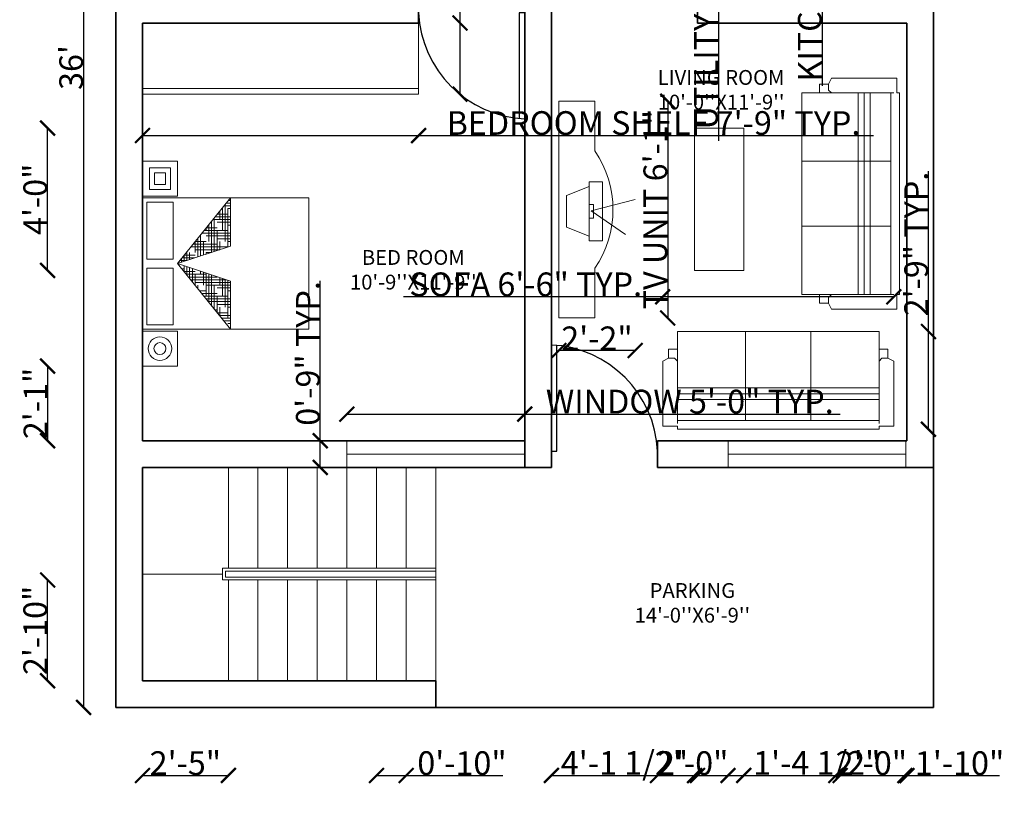
# Model space of a CAD drawing. Units: inches. Extents: x 2435 to 2891, y 1790 to 2334.
# Tile 1 of 3: x 2491 to 2823, y 1790 to 2052. Entities that reach past the tile are written whole.
import ezdxf

# ---------------------------------------------------------------- set-up
doc = ezdxf.new("R2010")
doc.units = ezdxf.units.IN
for name, color, linetype, lineweight in [('A-ANNO-DIMS', 2, 'Continuous', 13), ('A-AREA-IDEN', 7, 'Continuous', 18), ('A-FURN', 8, 'Continuous', 18), ('DOOR', 30, 'Continuous', 25), ('SHELF', 140, 'Continuous', 18), ('STEPS', 50, 'Continuous', 18), ('WALL', 7, 'Continuous', 35), ('WINDOW', 170, 'Continuous', 18)]:
    doc.layers.add(name, color=color, linetype=linetype, lineweight=lineweight)
doc.styles.get("Standard").update_dxf_attribs({"font": 'arial.ttf'})
doc.dimstyles.get("Standard").update_dxf_attribs({"dimtxt": 8, "dimasz": 5, "dimexe": 0.18, "dimexo": 0.0625, "dimgap": 0.09, "dimtad": 1, "dimdec": 1, "dimzin": 0, "dimdsep": 46, "dimlunit": 4, "dimtxsty": 'Standard', "dimblk": 'ARCHTICK', "dimcen": 0.09, "dimse1": 1, "dimse2": 1, "dimadec": 0, "dimazin": 0, "dimtfac": 1, "dimtdec": 1, "dimtofl": 0, "dimtmove": 0, "dimatfit": 3, "dimfxl": 1, "dimtolj": 1, "dimtzin": 0, "dimarcsym": 0})

# ---------------------------------------------------------------- blocks, each defined once
blk = doc.blocks.new('*X3')
at = {"color": 0}
for p, q in [((20.149, 14.719), (20.277, 14.719)), ((20.156, 14.625), (20.156, 14.728)), ((20.174, 14.75), (20.277, 14.75)), ((20.188, 14.75), (20.188, 14.767)), ((20.199, 14.781), (20.277, 14.781)), ((20.25, 14.812), (20.277, 14.812)), ((20.25, 14.319), (20.25, 14.75)), ((20.062, 14.257), (20.062, 14.612)), ((20.094, 14.375), (20.094, 14.65)), ((20.098, 14.656), (20.125, 14.656)), ((20.124, 14.688), (20.25, 14.688)), ((20.125, 14.5), (20.125, 14.689)), ((20.219, 14.309), (20.219, 14.625)), ((20.25, 14.625), (20.277, 14.625)), ((19.973, 14.5), (20.25, 14.5)), ((19.998, 14.531), (20.277, 14.531)), ((20, 14.237), (20, 14.5)), ((20.023, 14.562), (20.277, 14.562)), ((20.031, 14.247), (20.031, 14.573)), ((20.125, 14.594), (20.277, 14.594)), ((20.188, 14.299), (20.188, 14.5)), ((19.906, 14.375), (19.906, 14.417)), ((19.922, 14.438), (20, 14.438)), ((19.948, 14.469), (20.125, 14.469)), ((20.125, 14.406), (20.277, 14.406)), ((20.25, 14.438), (20.277, 14.438)), ((19.797, 14.281), (20.125, 14.281)), ((19.812, 14.174), (19.812, 14.301)), ((19.822, 14.312), (20.229, 14.312)), ((19.844, 14.185), (19.844, 14.34)), ((19.875, 14.25), (19.875, 14.379)), ((19.875, 14.344), (20.277, 14.344)), ((19.969, 14.226), (19.969, 14.375)), ((20, 14.375), (20.277, 14.375)), ((20.156, 14.288), (20.156, 14.375)), ((19.721, 14.188), (19.75, 14.188)), ((19.746, 14.219), (19.875, 14.219)), ((19.75, 14.154), (19.75, 14.223)), ((19.772, 14.25), (20, 14.25)), ((19.781, 14.164), (19.781, 14.262)), ((19.938, 14.216), (19.938, 14.25)), ((19.702, 14.094), (19.779, 14.094)), ((19.719, 14.073), (19.719, 14.114)), ((19.727, 14.062), (19.873, 14.062)), ((19.75, 14.034), (19.75, 14.103)), ((19.781, 13.995), (19.781, 14.093)), ((19.812, 14), (19.812, 14.082)), ((19.906, 13.84), (19.906, 14.051)), ((19.752, 14.031), (19.875, 14.031)), ((19.827, 13.938), (20.25, 13.938)), ((19.875, 13.878), (19.875, 14)), ((19.875, 13.969), (20.156, 13.969)), ((19.938, 13.801), (19.938, 14.041)), ((19.969, 13.875), (19.969, 14.031)), ((20, 14), (20, 14.02)), ((20, 14), (20.061, 14)), ((20.062, 13.645), (20.062, 14)), ((20.094, 13.625), (20.094, 13.989)), ((20.125, 13.75), (20.125, 13.979)), ((20.156, 13.875), (20.156, 13.969)), ((20.25, 13.5), (20.25, 13.937)), ((19.853, 13.906), (20.125, 13.906)), ((19.878, 13.875), (20, 13.875)), ((20.031, 13.684), (20.031, 13.875)), ((20.125, 13.844), (20.277, 13.844)), ((20.219, 13.451), (20.219, 13.875)), ((20.25, 13.875), (20.277, 13.875)), ((19.953, 13.781), (20.277, 13.781)), ((19.978, 13.75), (20.25, 13.75)), ((20, 13.812), (20.277, 13.812)), ((20, 13.723), (20, 13.75)), ((20.003, 13.719), (20.125, 13.719)), ((20.188, 13.49), (20.188, 13.75)), ((20.079, 13.625), (20.277, 13.625)), ((20.104, 13.594), (20.277, 13.594)), ((20.125, 13.656), (20.277, 13.656)), ((20.156, 13.529), (20.156, 13.625)), ((20.25, 13.688), (20.277, 13.688)), ((20.129, 13.562), (20.25, 13.562)), ((20.25, 13.5), (20.277, 13.5)), ((20.205, 13.469), (20.277, 13.469)), ((20.23, 13.438), (20.277, 13.438)), ((20.255, 13.406), (20.277, 13.406))]:
    blk.add_line(p, q, dxfattribs=at)
blk = doc.blocks.new('MAT-P13')
for p, q in [((-1.17, 0), (-1.17, -0.4)), ((-1.17, 0), (-0.77, 0)), ((-0.77, 0), (-0.77, -0.4)), ((-0.75, 0), (0.75, 0)), ((-0.75, 0), (-0.75, -1.9)), ((0.75, 0), (0.75, -1.9)), ((0.77, 0), (1.17, 0)), ((0.77, 0), (0.77, -0.4)), ((1.17, 0), (1.17, -0.4)), ((-0.7, -0.05), (-0.7, -0.35)), ((-0.7, -0.05), (-0.05, -0.05)), ((-0.05, -0.35), (-0.05, -0.05)), ((0.05, -0.05), (0.7, -0.05)), ((0.05, -0.35), (0.05, -0.05)), ((0.7, -0.05), (0.7, -0.35)), ((-1.17, -0.4), (-0.77, -0.4)), ((-0.75, -1.003), (0, -0.4)), ((0, -0.4), (-0.75, -1.003)), ((-0.7, -0.35), (-0.05, -0.35)), ((0, -0.4), (-0.2, -1.003)), ((0, -0.4), (0.2, -1.003)), ((0, -0.4), (0.75, -1.003)), ((0.05, -0.35), (0.7, -0.35)), ((0.77, -0.4), (1.17, -0.4)), ((-0.75, -1.003), (-0.2, -1.003)), ((0.2, -1.003), (0.75, -1.003)), ((0.75, -1.9), (-0.75, -1.9))]:
    blk.add_line(p, q)
for points in [[(0.847, -0.081), (1.093, -0.081), (1.093, -0.319), (0.847, -0.319)], [(0.902, -0.136), (1.038, -0.136), (1.038, -0.264), (0.902, -0.264)]]:
    blk.add_lwpolyline(points, close=True)
for radius in [0.134, 0.0686]:
    blk.add_circle((-0.97, -0.2), radius)
at = {"xscale": -1, "rotation": 90}
blk.add_blockref('*X3', (14.128, 19.274), dxfattribs=at)
blk = doc.blocks.new('12PCOU13')
at = {"color": 0, "linetype": 'ByBlock'}
for p, q in [((24, 37), (24, 35)), ((23, 34), (2, 34)), ((3, -34), (3, 34)), ((10, 34), (10, -34)), ((12, 34), (12, -34)), ((14, 34), (14, -34)), ((24, 35), (23, 34)), ((27, 34), (23, 34)), ((33, 11), (3, 11)), ((33, -11), (3, -11)), ((23, -34), (2, -34)), ((27, -34), (23, -34)), ((24, -35), (23, -34)), ((24, -37), (24, -35))]:
    blk.add_line(p, q, dxfattribs=at)
blk.add_lwpolyline([(1, -39), (1, -34), (0, -34), (0, 34), (1, 34), (1, 39), (23, 39), (24, 37), (27, 37), (27, 34), (33, 34), (33, -34), (27, -34), (27, -37), (24, -37), (23, -39)], close=True, dxfattribs=at)
blk = doc.blocks.new('AP0B05')
for p, q in [((35, 100), (35, 880)), ((75, 100), (75, 878.9)), ((35, 100), (35, -20)), ((815, 100), (815, -20))]:
    blk.add_line(p, q)
blk.add_lwpolyline([(35, 100), (75, 100)])
blk.add_arc((-2.4, 62.6), 818.3, 2.62122, 87.37878)
blk = doc.blocks.new('banghe81')
for p, q in [((-500, 3000), (0, 3000)), ((-500, 2312), (-500, 3000)), ((0, 3000), (0, 0)), ((-607, 1930), (-419, 1930)), ((-607, 1117), (-607, 1930)), ((-419, 1930), (-419, 1117)), ((-925, 1843), (-450, 1517)), ((-107, 1742), (-419, 1867)), ((-107, 1305), (-107, 1742)), ((-450, 1517), (-1057, 1361)), ((-482, 1617), (-482, 1430)), ((-419, 1617), (-482, 1617)), ((-482, 1430), (-419, 1430)), ((-419, 1180), (-107, 1305)), ((-419, 1117), (-607, 1117)), ((-500, 0), (-500, 688)), ((0, 0), (-500, 0)), ((-500, 0), (-500, 0))]:
    blk.add_line(p, q)
blk.add_arc((695, 1500), 1445, 145.7945, 214.2055)
blk = doc.blocks.new('_ArchTick')
at = {"color": 0, "linetype": 'ByBlock', "const_width": 0.15}
blk.add_lwpolyline([(-0.5, -0.5), (0.5, 0.5)], dxfattribs=at)
blk = doc.blocks.new('*D11')
at = {"layer": 'A-ANNO-DIMS', "color": 0, "lineweight": -2, "transparency": 16777216}
blk.add_line((2512.57, 2252.2), (2512.57, 1820.2), dxfattribs=at)
at = {"layer": 'Defpoints', "color": 0, "transparency": 16777216}
for p in [(2523.44, 2252.2), (2512.57, 1820.2), (2523.44, 1820.2)]:
    blk.add_point(p, dxfattribs=at)
at = {"layer": 'A-ANNO-DIMS', "color": 0, "lineweight": -2, "transparency": 16777216, "xscale": 5, "yscale": 5, "zscale": 5}
for p, rotation in [((2512.57, 2252.2), 90), ((2512.57, 1820.2), 270)]:
    blk.add_blockref('_ArchTick', p, dxfattribs=dict(at, rotation=rotation))
at = {"layer": 'A-ANNO-DIMS', "color": 0, "transparency": 16777216, "insert": (2508.39, 2036.2), "char_height": 8, "attachment_point": 5, "rotation": 90}
blk.add_mtext("\\A1;36'", dxfattribs=at)
blk = doc.blocks.new('WIN-60IN')
blk.add_line((0, 4.5), (60, 4.5))
blk.add_lwpolyline([(0, 9), (60, 9), (60, 0), (0, 0)], close=True)
blk = doc.blocks.new('SHELF-BEDROOM')
for p, q in [((93.19, 0), (93.19, 24)), ((0, 1.9), (93.19, 1.9)), ((0, 0), (93.19, 0))]:
    blk.add_line(p, q)
blk = doc.blocks.new('*D17')
at = {"layer": 'A-ANNO-DIMS', "color": 0, "lineweight": -2, "transparency": 16777216}
for p, q in [((2726.86, 2213.2), (2726.86, 2166.02)), ((2726.86, 2166.02), (2726.86, 2011.45))]:
    blk.add_line(p, q, dxfattribs=at)
at = {"layer": 'Defpoints', "color": 0, "transparency": 16777216}
for p in [(2719.78, 2213.2), (2719.78, 2166.02), (2726.86, 2166.02)]:
    blk.add_point(p, dxfattribs=at)
at = {"layer": 'A-ANNO-DIMS', "color": 0, "lineweight": -2, "transparency": 16777216, "xscale": 5, "yscale": 5, "zscale": 5}
for p, rotation in [((2726.86, 2213.2), 90), ((2726.86, 2166.02), 270)]:
    blk.add_blockref('_ArchTick', p, dxfattribs=dict(at, rotation=rotation))
at = {"layer": 'A-ANNO-DIMS', "color": 0, "transparency": 16777216, "insert": (2722.63, 2086.24), "char_height": 8, "attachment_point": 5, "rotation": 90}
blk.add_mtext('\\A1;UTILITY DOOR SWING 3\'-11"', dxfattribs=at)
blk = doc.blocks.new('*D21')
at = {"layer": 'A-ANNO-DIMS', "color": 0, "lineweight": -2, "transparency": 16777216}
for p, q in [((2601.44, 1919.2), (2661.44, 1919.2)), ((2661.44, 1919.2), (2767.86, 1919.2))]:
    blk.add_line(p, q, dxfattribs=at)
at = {"layer": 'Defpoints', "color": 0, "transparency": 16777216}
for p in [(2661.44, 1919.2), (2601.44, 1910.2), (2661.44, 1910.2)]:
    blk.add_point(p, dxfattribs=at)
at = {"layer": 'A-ANNO-DIMS', "color": 0, "lineweight": -2, "transparency": 16777216, "xscale": 5, "yscale": 5, "zscale": 5, "rotation": 180}
blk.add_blockref('_ArchTick', (2601.44, 1919.2), dxfattribs=at)
at = {"layer": 'A-ANNO-DIMS', "color": 0, "lineweight": -2, "transparency": 16777216, "xscale": 5, "yscale": 5, "zscale": 5}
blk.add_blockref('_ArchTick', (2661.44, 1919.2), dxfattribs=at)
at = {"layer": 'A-ANNO-DIMS', "color": 0, "transparency": 16777216, "insert": (2717.15, 1923.43), "char_height": 8, "attachment_point": 5}
blk.add_mtext('\\A1;WINDOW 5\'-0" TYP.', dxfattribs=at)
blk = doc.blocks.new('*D22')
at = {"layer": 'A-ANNO-DIMS', "color": 0, "lineweight": -2, "transparency": 16777216}
for p, q in [((2592.44, 1910.2), (2592.44, 1964.15)), ((2592.44, 1901.2), (2592.44, 1910.2))]:
    blk.add_line(p, q, dxfattribs=at)
at = {"layer": 'Defpoints', "color": 0, "transparency": 16777216}
for p in [(2592.44, 1910.2), (2601.44, 1910.2), (2601.44, 1901.2)]:
    blk.add_point(p, dxfattribs=at)
at = {"layer": 'A-ANNO-DIMS', "color": 0, "lineweight": -2, "transparency": 16777216, "xscale": 5, "yscale": 5, "zscale": 5}
for p, rotation in [((2592.44, 1910.2), 90), ((2592.44, 1901.2), 270)]:
    blk.add_blockref('_ArchTick', p, dxfattribs=dict(at, rotation=rotation))
at = {"layer": 'A-ANNO-DIMS', "color": 0, "transparency": 16777216, "insert": (2588.27, 1939.68), "char_height": 8, "attachment_point": 5, "rotation": 90}
blk.add_mtext('\\A1;0\'-9" TYP.', dxfattribs=at)
blk = doc.blocks.new('*D25')
at = {"layer": 'A-ANNO-DIMS', "color": 0, "lineweight": -2, "transparency": 16777216}
for p, q in [((2708.01, 1958.78), (2620.57, 1958.78)), ((2786.01, 1958.78), (2708.01, 1958.78))]:
    blk.add_line(p, q, dxfattribs=at)
at = {"layer": 'Defpoints', "color": 0, "transparency": 16777216}
for p in [(2708.01, 1958.78), (2708.01, 1947.08), (2786.01, 1947.08)]:
    blk.add_point(p, dxfattribs=at)
at = {"layer": 'A-ANNO-DIMS', "color": 0, "lineweight": -2, "transparency": 16777216, "xscale": 5, "yscale": 5, "zscale": 5, "rotation": 180}
blk.add_blockref('_ArchTick', (2708.01, 1958.78), dxfattribs=at)
at = {"layer": 'A-ANNO-DIMS', "color": 0, "lineweight": -2, "transparency": 16777216, "xscale": 5, "yscale": 5, "zscale": 5}
blk.add_blockref('_ArchTick', (2786.01, 1958.78), dxfattribs=at)
at = {"layer": 'A-ANNO-DIMS', "color": 0, "transparency": 16777216, "insert": (2661.79, 1963.01), "char_height": 8, "attachment_point": 5}
blk.add_mtext('\\A1;SOFA 6\'-6" TYP.', dxfattribs=at)
blk = doc.blocks.new('*D26')
at = {"layer": 'A-ANNO-DIMS', "color": 0, "lineweight": -2, "transparency": 16777216}
for p, q in [((2797.71, 1947.08), (2797.71, 2001.16)), ((2797.71, 1914.08), (2797.71, 1947.08))]:
    blk.add_line(p, q, dxfattribs=at)
at = {"layer": 'Defpoints', "color": 0, "transparency": 16777216}
for p in [(2786.01, 1947.08), (2797.71, 1947.08), (2786.01, 1914.08)]:
    blk.add_point(p, dxfattribs=at)
at = {"layer": 'A-ANNO-DIMS', "color": 0, "lineweight": -2, "transparency": 16777216, "xscale": 5, "yscale": 5, "zscale": 5}
for p, rotation in [((2797.71, 1947.08), 90), ((2797.71, 1914.08), 270)]:
    blk.add_blockref('_ArchTick', p, dxfattribs=dict(at, rotation=rotation))
at = {"layer": 'A-ANNO-DIMS', "color": 0, "transparency": 16777216, "insert": (2793.53, 1976.62), "char_height": 8, "attachment_point": 5, "rotation": 90}
blk.add_mtext('\\A1;2\'-9" TYP.', dxfattribs=at)
blk = doc.blocks.new('*D27')
at = {"layer": 'A-ANNO-DIMS', "color": 0, "lineweight": -2, "transparency": 16777216}
for p, q in [((2532.44, 2013.23), (2625.63, 2013.23)), ((2625.63, 2013.23), (2779.2, 2013.23))]:
    blk.add_line(p, q, dxfattribs=at)
at = {"layer": 'Defpoints', "color": 0, "transparency": 16777216}
for p in [(2532.44, 2027.2), (2625.63, 2027.2), (2625.63, 2013.23)]:
    blk.add_point(p, dxfattribs=at)
at = {"layer": 'A-ANNO-DIMS', "color": 0, "lineweight": -2, "transparency": 16777216, "xscale": 5, "yscale": 5, "zscale": 5, "rotation": 180}
blk.add_blockref('_ArchTick', (2532.44, 2013.23), dxfattribs=at)
at = {"layer": 'A-ANNO-DIMS', "color": 0, "lineweight": -2, "transparency": 16777216, "xscale": 5, "yscale": 5, "zscale": 5}
blk.add_blockref('_ArchTick', (2625.63, 2013.23), dxfattribs=at)
at = {"layer": 'A-ANNO-DIMS', "color": 0, "transparency": 16777216, "insert": (2704.91, 2017.46), "char_height": 8, "attachment_point": 5}
blk.add_mtext('\\A1;BEDROOM SHELF 7\'-9" TYP.', dxfattribs=at)
blk = doc.blocks.new('*D28')
at = {"layer": 'A-ANNO-DIMS', "color": 0, "lineweight": -2, "transparency": 16777216}
for p, q in [((2639.61, 2051.2), (2639.61, 2105.28)), ((2639.61, 2027.2), (2639.61, 2051.2))]:
    blk.add_line(p, q, dxfattribs=at)
at = {"layer": 'Defpoints', "color": 0, "transparency": 16777216}
for p in [(2625.63, 2051.2), (2639.61, 2051.2), (2625.63, 2027.2)]:
    blk.add_point(p, dxfattribs=at)
at = {"layer": 'A-ANNO-DIMS', "color": 0, "lineweight": -2, "transparency": 16777216, "xscale": 5, "yscale": 5, "zscale": 5}
for p, rotation in [((2639.61, 2051.2), 90), ((2639.61, 2027.2), 270)]:
    blk.add_blockref('_ArchTick', p, dxfattribs=dict(at, rotation=rotation))
at = {"layer": 'A-ANNO-DIMS', "color": 0, "transparency": 16777216, "insert": (2635.43, 2080.74), "char_height": 8, "attachment_point": 5, "rotation": 90}
blk.add_mtext('\\A1;2\'-0" TYP.', dxfattribs=at)
blk = doc.blocks.new('*D31')
at = {"layer": 'A-ANNO-DIMS', "color": 0, "lineweight": -2, "transparency": 16777216}
for p, q in [((2761.88, 2181.68), (2761.88, 2137.5)), ((2761.88, 2137.5), (2761.88, 2030.06))]:
    blk.add_line(p, q, dxfattribs=at)
at = {"layer": 'Defpoints', "color": 0, "transparency": 16777216}
for p in [(2768.5, 2181.68), (2761.88, 2137.5), (2768.5, 2137.5)]:
    blk.add_point(p, dxfattribs=at)
at = {"layer": 'A-ANNO-DIMS', "color": 0, "lineweight": -2, "transparency": 16777216, "xscale": 5, "yscale": 5, "zscale": 5}
for p, rotation in [((2761.88, 2181.68), 90), ((2761.88, 2137.5), 270)]:
    blk.add_blockref('_ArchTick', p, dxfattribs=dict(at, rotation=rotation))
at = {"layer": 'A-ANNO-DIMS', "color": 0, "transparency": 16777216, "insert": (2757.65, 2081.28), "char_height": 8, "attachment_point": 5, "rotation": 90}
blk.add_mtext('\\A1;KITCHEN SINK 3\'-8"', dxfattribs=at)
blk = doc.blocks.new('*D33')
at = {"layer": 'A-ANNO-DIMS', "color": 0, "lineweight": -2, "transparency": 16777216}
blk.add_line((2709.7, 2024.82), (2709.7, 1951.65), dxfattribs=at)
at = {"layer": 'Defpoints', "color": 0, "transparency": 16777216}
for p in [(2698.72, 2024.82), (2698.72, 1951.65), (2709.7, 1951.65)]:
    blk.add_point(p, dxfattribs=at)
at = {"layer": 'A-ANNO-DIMS', "color": 0, "lineweight": -2, "transparency": 16777216, "xscale": 5, "yscale": 5, "zscale": 5}
for p, rotation in [((2709.7, 2024.82), 90), ((2709.7, 1951.65), 270)]:
    blk.add_blockref('_ArchTick', p, dxfattribs=dict(at, rotation=rotation))
at = {"layer": 'A-ANNO-DIMS', "color": 0, "transparency": 16777216, "insert": (2705.52, 1988.23), "char_height": 8, "attachment_point": 5, "rotation": 90}
blk.add_mtext('\\A1;TV UNIT 6\'-1"', dxfattribs=at)
blk = doc.blocks.new('*D34')
at = {"layer": 'A-ANNO-DIMS', "color": 0, "lineweight": -2, "transparency": 16777216}
blk.add_line((2698.72, 1940.67), (2672.94, 1940.67), dxfattribs=at)
at = {"layer": 'Defpoints', "color": 0, "transparency": 16777216}
for p in [(2672.94, 1951.65), (2698.72, 1951.65), (2672.94, 1940.67)]:
    blk.add_point(p, dxfattribs=at)
at = {"layer": 'A-ANNO-DIMS', "color": 0, "lineweight": -2, "transparency": 16777216, "xscale": 5, "yscale": 5, "zscale": 5, "rotation": 180}
blk.add_blockref('_ArchTick', (2672.94, 1940.67), dxfattribs=at)
at = {"layer": 'A-ANNO-DIMS', "color": 0, "lineweight": -2, "transparency": 16777216, "xscale": 5, "yscale": 5, "zscale": 5}
blk.add_blockref('_ArchTick', (2698.72, 1940.67), dxfattribs=at)
at = {"layer": 'A-ANNO-DIMS', "color": 0, "transparency": 16777216, "insert": (2685.83, 1944.78), "char_height": 8, "attachment_point": 5}
blk.add_mtext('\\A1;2\'-2"', dxfattribs=at)
blk = doc.blocks.new('*D41')
at = {"layer": 'A-ANNO-DIMS', "color": 0, "lineweight": -2, "transparency": 16777216}
blk.add_line((2532.44, 1797.2), (2561.44, 1797.2), dxfattribs=at)
at = {"layer": 'Defpoints', "color": 0, "transparency": 16777216}
for p in [(2532.44, 1829.2), (2561.44, 1829.2), (2561.44, 1797.2)]:
    blk.add_point(p, dxfattribs=at)
at = {"layer": 'A-ANNO-DIMS', "color": 0, "lineweight": -2, "transparency": 16777216, "xscale": 5, "yscale": 5, "zscale": 5, "rotation": 180}
blk.add_blockref('_ArchTick', (2532.44, 1797.2), dxfattribs=at)
at = {"layer": 'A-ANNO-DIMS', "color": 0, "lineweight": -2, "transparency": 16777216, "xscale": 5, "yscale": 5, "zscale": 5}
blk.add_blockref('_ArchTick', (2561.44, 1797.2), dxfattribs=at)
at = {"layer": 'A-ANNO-DIMS', "color": 0, "transparency": 16777216, "insert": (2546.94, 1801.38), "char_height": 8, "attachment_point": 5}
blk.add_mtext('\\A1;2\'-5"', dxfattribs=at)
blk = doc.blocks.new('*D42')
at = {"layer": 'A-ANNO-DIMS', "color": 0, "lineweight": -2, "transparency": 16777216}
for p, q in [((2611.44, 1797.2), (2621.44, 1797.2)), ((2621.44, 1797.2), (2654.11, 1797.2))]:
    blk.add_line(p, q, dxfattribs=at)
at = {"layer": 'Defpoints', "color": 0, "transparency": 16777216}
for p in [(2611.44, 1829.2), (2621.44, 1829.2), (2621.44, 1797.2)]:
    blk.add_point(p, dxfattribs=at)
at = {"layer": 'A-ANNO-DIMS', "color": 0, "lineweight": -2, "transparency": 16777216, "xscale": 5, "yscale": 5, "zscale": 5, "rotation": 180}
blk.add_blockref('_ArchTick', (2611.44, 1797.2), dxfattribs=at)
at = {"layer": 'A-ANNO-DIMS', "color": 0, "lineweight": -2, "transparency": 16777216, "xscale": 5, "yscale": 5, "zscale": 5}
blk.add_blockref('_ArchTick', (2621.44, 1797.2), dxfattribs=at)
at = {"layer": 'A-ANNO-DIMS', "color": 0, "transparency": 16777216, "insert": (2640.28, 1801.38), "char_height": 8, "attachment_point": 5}
blk.add_mtext('\\A1;0\'-10"', dxfattribs=at)
blk = doc.blocks.new('*D43')
at = {"layer": 'A-ANNO-DIMS', "color": 0, "lineweight": -2, "transparency": 16777216}
blk.add_line((2500.44, 1829.2), (2500.44, 1863.2), dxfattribs=at)
at = {"layer": 'Defpoints', "color": 0, "transparency": 16777216}
for p in [(2500.44, 1863.2), (2561.44, 1863.2), (2561.44, 1829.2)]:
    blk.add_point(p, dxfattribs=at)
at = {"layer": 'A-ANNO-DIMS', "color": 0, "lineweight": -2, "transparency": 16777216, "xscale": 5, "yscale": 5, "zscale": 5}
for p, rotation in [((2500.44, 1863.2), 90), ((2500.44, 1829.2), 270)]:
    blk.add_blockref('_ArchTick', p, dxfattribs=dict(at, rotation=rotation))
at = {"layer": 'A-ANNO-DIMS', "color": 0, "transparency": 16777216, "insert": (2496.27, 1846.2), "char_height": 8, "attachment_point": 5, "rotation": 90}
blk.add_mtext('\\A1;2\'-10"', dxfattribs=at)
blk = doc.blocks.new('*D44')
at = {"layer": 'A-ANNO-DIMS', "color": 0, "lineweight": -2, "transparency": 16777216}
blk.add_line((2706.26, 1797.2), (2730.05, 1797.2), dxfattribs=at)
at = {"layer": 'Defpoints', "color": 0, "transparency": 16777216}
for p in [(2706.26, 1901.2), (2730.05, 1901.2), (2730.05, 1797.2)]:
    blk.add_point(p, dxfattribs=at)
at = {"layer": 'A-ANNO-DIMS', "color": 0, "lineweight": -2, "transparency": 16777216, "xscale": 5, "yscale": 5, "zscale": 5, "rotation": 180}
blk.add_blockref('_ArchTick', (2706.26, 1797.2), dxfattribs=at)
at = {"layer": 'A-ANNO-DIMS', "color": 0, "lineweight": -2, "transparency": 16777216, "xscale": 5, "yscale": 5, "zscale": 5}
blk.add_blockref('_ArchTick', (2730.05, 1797.2), dxfattribs=at)
at = {"layer": 'A-ANNO-DIMS', "color": 0, "transparency": 16777216, "insert": (2718.15, 1801.38), "char_height": 8, "attachment_point": 5}
blk.add_mtext('\\A1;2\'-0"', dxfattribs=at)
blk = doc.blocks.new('*D47')
at = {"layer": 'A-ANNO-DIMS', "color": 0, "lineweight": -2, "transparency": 16777216}
blk.add_line((2670.44, 1797.2), (2719.78, 1797.2), dxfattribs=at)
at = {"layer": 'Defpoints', "color": 0, "transparency": 16777216}
for p in [(2670.44, 2060.2), (2719.78, 2060.2), (2719.78, 1797.2)]:
    blk.add_point(p, dxfattribs=at)
at = {"layer": 'A-ANNO-DIMS', "color": 0, "lineweight": -2, "transparency": 16777216, "xscale": 5, "yscale": 5, "zscale": 5, "rotation": 180}
blk.add_blockref('_ArchTick', (2670.44, 1797.2), dxfattribs=at)
at = {"layer": 'A-ANNO-DIMS', "color": 0, "lineweight": -2, "transparency": 16777216, "xscale": 5, "yscale": 5, "zscale": 5}
blk.add_blockref('_ArchTick', (2719.78, 1797.2), dxfattribs=at)
at = {"layer": 'A-ANNO-DIMS', "color": 0, "transparency": 16777216, "insert": (2695.11, 1801.43), "char_height": 8, "attachment_point": 5}
blk.add_mtext('\\A1;4\'-1 1/2"', dxfattribs=at)
blk = doc.blocks.new('*D48')
at = {"layer": 'A-ANNO-DIMS', "color": 0, "lineweight": -2, "transparency": 16777216}
blk.add_line((2766.44, 1797.2), (2790.44, 1797.2), dxfattribs=at)
at = {"layer": 'Defpoints', "color": 0, "transparency": 16777216}
for p in [(2766.44, 2060.2), (2790.44, 2060.2), (2790.44, 1797.2)]:
    blk.add_point(p, dxfattribs=at)
at = {"layer": 'A-ANNO-DIMS', "color": 0, "lineweight": -2, "transparency": 16777216, "xscale": 5, "yscale": 5, "zscale": 5, "rotation": 180}
blk.add_blockref('_ArchTick', (2766.44, 1797.2), dxfattribs=at)
at = {"layer": 'A-ANNO-DIMS', "color": 0, "lineweight": -2, "transparency": 16777216, "xscale": 5, "yscale": 5, "zscale": 5}
blk.add_blockref('_ArchTick', (2790.44, 1797.2), dxfattribs=at)
at = {"layer": 'A-ANNO-DIMS', "color": 0, "transparency": 16777216, "insert": (2778.44, 1801.38), "char_height": 8, "attachment_point": 5}
blk.add_mtext('\\A1;2\'-0"', dxfattribs=at)
blk = doc.blocks.new('*D53')
at = {"layer": 'A-ANNO-DIMS', "color": 0, "lineweight": -2, "transparency": 16777216}
for p, q in [((2767.88, 1797.2), (2789.76, 1797.2)), ((2789.76, 1797.2), (2821.66, 1797.2))]:
    blk.add_line(p, q, dxfattribs=at)
at = {"layer": 'Defpoints', "color": 0, "transparency": 16777216}
for p in [(2767.88, 2102.71), (2789.76, 2102.71), (2789.76, 1797.2)]:
    blk.add_point(p, dxfattribs=at)
at = {"layer": 'A-ANNO-DIMS', "color": 0, "lineweight": -2, "transparency": 16777216, "xscale": 5, "yscale": 5, "zscale": 5, "rotation": 180}
blk.add_blockref('_ArchTick', (2767.88, 1797.2), dxfattribs=at)
at = {"layer": 'A-ANNO-DIMS', "color": 0, "lineweight": -2, "transparency": 16777216, "xscale": 5, "yscale": 5, "zscale": 5}
blk.add_blockref('_ArchTick', (2789.76, 1797.2), dxfattribs=at)
at = {"layer": 'A-ANNO-DIMS', "color": 0, "transparency": 16777216, "insert": (2808.21, 1801.38), "char_height": 8, "attachment_point": 5}
blk.add_mtext('\\A1;1\'-10"', dxfattribs=at)
blk = doc.blocks.new('*D55')
at = {"layer": 'A-ANNO-DIMS', "color": 0, "lineweight": -2, "transparency": 16777216}
for p, q in [((2718.79, 1797.2), (2735.35, 1797.2)), ((2735.35, 1797.2), (2779.68, 1797.2))]:
    blk.add_line(p, q, dxfattribs=at)
at = {"layer": 'Defpoints', "color": 0, "transparency": 16777216}
for p in [(2718.79, 1967.71), (2735.35, 1967.71), (2735.35, 1797.2)]:
    blk.add_point(p, dxfattribs=at)
at = {"layer": 'A-ANNO-DIMS', "color": 0, "lineweight": -2, "transparency": 16777216, "xscale": 5, "yscale": 5, "zscale": 5, "rotation": 180}
blk.add_blockref('_ArchTick', (2718.79, 1797.2), dxfattribs=at)
at = {"layer": 'A-ANNO-DIMS', "color": 0, "lineweight": -2, "transparency": 16777216, "xscale": 5, "yscale": 5, "zscale": 5}
blk.add_blockref('_ArchTick', (2735.35, 1797.2), dxfattribs=at)
at = {"layer": 'A-ANNO-DIMS', "color": 0, "transparency": 16777216, "insert": (2760.01, 1801.43), "char_height": 8, "attachment_point": 5}
blk.add_mtext('\\A1;1\'-4 1/2"', dxfattribs=at)
blk = doc.blocks.new('*D56')
at = {"layer": 'A-ANNO-DIMS', "color": 0, "lineweight": -2, "transparency": 16777216}
blk.add_line((2500.44, 1967.71), (2500.44, 2015.75), dxfattribs=at)
at = {"layer": 'Defpoints', "color": 0, "transparency": 16777216}
for p in [(2500.44, 2015.75), (2718.79, 2015.75), (2718.79, 1967.71)]:
    blk.add_point(p, dxfattribs=at)
at = {"layer": 'A-ANNO-DIMS', "color": 0, "lineweight": -2, "transparency": 16777216, "xscale": 5, "yscale": 5, "zscale": 5}
for p, rotation in [((2500.44, 2015.75), 90), ((2500.44, 1967.71), 270)]:
    blk.add_blockref('_ArchTick', p, dxfattribs=dict(at, rotation=rotation))
at = {"layer": 'A-ANNO-DIMS', "color": 0, "transparency": 16777216, "insert": (2496.27, 1991.73), "char_height": 8, "attachment_point": 5, "rotation": 90}
blk.add_mtext('\\A1;4\'-0"', dxfattribs=at)
blk = doc.blocks.new('*D57')
at = {"layer": 'A-ANNO-DIMS', "color": 0, "lineweight": -2, "transparency": 16777216}
blk.add_line((2500.44, 1935.4), (2500.44, 1910.2), dxfattribs=at)
at = {"layer": 'Defpoints', "color": 0, "transparency": 16777216}
for p in [(2532.44, 1935.4), (2500.44, 1910.2), (2532.44, 1910.2)]:
    blk.add_point(p, dxfattribs=at)
at = {"layer": 'A-ANNO-DIMS', "color": 0, "lineweight": -2, "transparency": 16777216, "xscale": 5, "yscale": 5, "zscale": 5}
for p, rotation in [((2500.44, 1935.4), 90), ((2500.44, 1910.2), 270)]:
    blk.add_blockref('_ArchTick', p, dxfattribs=dict(at, rotation=rotation))
at = {"layer": 'A-ANNO-DIMS', "color": 0, "transparency": 16777216, "insert": (2496.34, 1922.8), "char_height": 8, "attachment_point": 5, "rotation": 90}
blk.add_mtext('\\A1;2\'-1"', dxfattribs=at)

msp = doc.modelspace()

# ---------------------------------------------------------------- linework, layer by layer
at = {"layer": 'A-FURN'}
msp.add_lwpolyline([(2718.79, 2015.75), (2735.35, 2015.75), (2735.35, 1967.71), (2718.79, 1967.71)], close=True, dxfattribs=at)
at = {"layer": 'STEPS'}
for p, q in [((2561.44, 1867.2), (2561.44, 1901.2)), ((2571.44, 1867.2), (2571.44, 1901.2)), ((2581.44, 1867.2), (2581.44, 1901.2)), ((2591.44, 1867.2), (2591.44, 1901.2)), ((2601.44, 1867.2), (2601.44, 1901.2)), ((2611.44, 1867.2), (2611.44, 1901.2)), ((2621.44, 1867.2), (2621.44, 1901.2)), ((2631.44, 1829.2), (2631.44, 1901.2)), ((2559.44, 1865.2), (2532.44, 1865.2)), ((2631.44, 1867.2), (2559.44, 1867.2)), ((2559.44, 1863.2), (2559.44, 1867.2)), ((2631.44, 1866.2), (2560.44, 1866.2)), ((2560.44, 1864.2), (2560.44, 1866.2)), ((2631.44, 1864.2), (2560.44, 1864.2)), ((2631.44, 1863.2), (2559.44, 1863.2)), ((2561.44, 1829.2), (2561.44, 1863.2)), ((2571.44, 1829.2), (2571.44, 1863.2)), ((2581.44, 1829.2), (2581.44, 1863.2)), ((2591.44, 1829.2), (2591.44, 1863.2)), ((2601.44, 1829.2), (2601.44, 1863.2)), ((2611.44, 1829.2), (2611.44, 1863.2)), ((2621.44, 1829.2), (2621.44, 1863.2))]:
    msp.add_line(p, q, dxfattribs=at)
at = {"layer": 'WALL'}
for p, q in [((2523.44, 2252.2), (2523.44, 1820.2)), ((2799.44, 2252.2), (2799.44, 1820.2)), ((2625.63, 2060.2), (2625.63, 2051.2)), ((2661.44, 2060.2), (2661.44, 1901.2)), ((2670.44, 2060.2), (2670.44, 1901.2)), ((2719.78, 2060.2), (2719.78, 2051.2)), ((2532.44, 2051.2), (2625.63, 2051.2)), ((2532.44, 2051.2), (2532.44, 1910.2)), ((2719.78, 2051.2), (2790.44, 2051.2)), ((2790.44, 2051.2), (2790.44, 1910.2)), ((2532.44, 1910.2), (2661.44, 1910.2)), ((2706.26, 1910.2), (2706.26, 1901.2)), ((2706.26, 1910.2), (2790.44, 1910.2)), ((2532.44, 1901.2), (2532.44, 1829.2)), ((2532.44, 1901.2), (2670.44, 1901.2)), ((2706.26, 1901.2), (2799.44, 1901.2)), ((2631.44, 1829.2), (2532.44, 1829.2)), ((2631.44, 1820.2), (2631.44, 1829.2)), ((2523.44, 1820.2), (2799.44, 1820.2))]:
    msp.add_line(p, q, dxfattribs=at)

# ---------------------------------------------------------------- block references
at = {"layer": 'A-FURN'}
for p, rotation in [((2787.98, 1993.6), 180), ((2747.01, 1914.08), 89.99999999999999)]:
    msp.add_blockref('12PCOU13', p, dxfattribs=dict(at, rotation=rotation))
for name, p, xscale, yscale, zscale, rotation in [('banghe81', (2672.94, 2024.82), 0.0243899890610312, 0.0243899890610312, 0.0243899890610312, 180), ('MAT-P13', (2532.44, 1970), 29.57686120969658, 29.57686120969658, 29.57686120969658, 90)]:
    msp.add_blockref(name, p, dxfattribs=dict(at, xscale=xscale, yscale=yscale, zscale=zscale, rotation=rotation))
at = {"layer": 'DOOR', "xscale": 0.0459165349072538, "yscale": 0.0459165349072538, "zscale": 0.0459165349072538, "rotation": 180}
msp.add_blockref('AP0B05', (2663.05, 2059.29), dxfattribs=at)
at = {"layer": 'DOOR', "xscale": 0.0459143749097, "yscale": 0.0459143749097, "zscale": 0.0459143749097}
msp.add_blockref('AP0B05', (2668.84, 1902.12), dxfattribs=at)
at = {"layer": 'SHELF'}
msp.add_blockref('SHELF-BEDROOM', (2532.44, 2027.2), dxfattribs=at)
at = {"layer": 'WINDOW'}
for p in [(2601.44, 1901.2), (2730.05, 1901.2)]:
    msp.add_blockref('WIN-60IN', p, dxfattribs=at)

# ---------------------------------------------------------------- texts
at = {"layer": 'A-AREA-IDEN', "char_height": 5, "attachment_point": 1}
for s, width, insert in [("\\pxqc;LIVING ROOM\\P10'-0''X11'-9''", 59.5406, (2697.95, 2035.35)), ("\\pxqc;BED ROOM\\P10'-9''X11'-9''", 37.2819, (2605.22, 1974.59)), ("\\pxqc;PARKING\\P14'-0''X6'-9''", 37.2819, (2699.39, 1862.15))]:
    msp.add_mtext_dynamic_manual_height_columns(s, width=width, gutter_width=12.5, heights=[0], dxfattribs=dict(at, insert=insert))

# ---------------------------------------------------------------- dimensions: what is measured, and where the dimension line sits
at = {"layer": 'A-ANNO-DIMS'}
for base, p1, p2, angle, override, picture, middle in [((2512.57, 1820.2), (2523.44, 2252.2), (2523.44, 1820.2), 90, {"dimclrd": 0, "dimclre": 0, "dimclrt": 0}, '*D11', (2508.39, 2036.2)), ((2500.44, 2015.75), (2718.79, 1967.71), (2718.79, 2015.75), 90, {"dimdec": 1, "dimlfac": 1, "dimrnd": 0, "dimzin": 1, "dimdsep": 46, "dimlunit": 4, "dimfrac": 2}, '*D56', (2496.27, 1991.73)), ((2672.94, 1940.67), (2698.72, 1951.65), (2672.94, 1951.65), 180, {"dimdec": 1, "dimlfac": 1, "dimrnd": 0, "dimzin": 1, "dimdsep": 46, "dimlunit": 4, "dimfrac": 2}, '*D34', (2685.83, 1944.78)), ((2500.44, 1910.2), (2532.44, 1935.4), (2532.44, 1910.2), 90, {"dimdec": 1, "dimlfac": 1, "dimrnd": 0, "dimzin": 1, "dimdsep": 46, "dimlunit": 4, "dimfrac": 2}, '*D57', (2496.34, 1922.8)), ((2500.44, 1863.2), (2561.44, 1829.2), (2561.44, 1863.2), 90, {"dimdec": 1, "dimlfac": 1, "dimrnd": 0, "dimzin": 1, "dimdsep": 46, "dimlunit": 4, "dimfrac": 2}, '*D43', (2496.27, 1846.2))]:
    dim = msp.add_linear_dim(base=base, p1=p1, p2=p2, angle=angle, dimstyle='Standard', override=override, dxfattribs=at)
    dim.commit()
    dim.dimension.update_dxf_attribs({"geometry": picture, "text_midpoint": middle})
for base, p1, p2, angle, text, picture, middle in [((2726.86, 2166.02), (2719.78, 2213.2), (2719.78, 2166.02), 270, 'UTILITY DOOR SWING <>', '*D17', (2722.63, 2086.24)), ((2761.88, 2137.5), (2768.5, 2181.68), (2768.5, 2137.5), 270, 'KITCHEN SINK <>', '*D31', (2757.65, 2081.28)), ((2639.61, 2051.2), (2625.63, 2027.2), (2625.63, 2051.2), 90, '<> TYP.', '*D28', (2635.43, 2080.74)), ((2709.7, 1951.65), (2698.72, 2024.82), (2698.72, 1951.65), 270, 'TV UNIT <>', '*D33', (2705.52, 1988.23)), ((2797.71, 1947.08), (2786.01, 1914.08), (2786.01, 1947.08), 90, '<> TYP.', '*D26', (2793.53, 1976.62)), ((2708.01, 1958.78), (2786.01, 1947.08), (2708.01, 1947.08), 180, 'SOFA <> TYP.', '*D25', (2661.79, 1963.01)), ((2592.44, 1910.2), (2601.44, 1901.2), (2601.44, 1910.2), 90, '<> TYP.', '*D22', (2588.27, 1939.68))]:
    dim = msp.add_linear_dim(base=base, p1=p1, p2=p2, angle=angle, text=text, dimstyle='Standard', override={"dimdec": 1, "dimlfac": 1, "dimrnd": 0, "dimzin": 1, "dimdsep": 46, "dimlunit": 4, "dimfrac": 2}, dxfattribs=at)
    dim.commit()
    dim.dimension.update_dxf_attribs({"geometry": picture, "text_midpoint": middle})
for base, p1, p2, picture, middle in [((2789.76, 1797.2), (2767.88, 2102.71), (2789.76, 2102.71), '*D53', (2808.21, 1801.38)), ((2719.78, 1797.2), (2670.44, 2060.2), (2719.78, 2060.2), '*D47', (2695.11, 1801.43)), ((2790.44, 1797.2), (2766.44, 2060.2), (2790.44, 2060.2), '*D48', (2778.44, 1801.38)), ((2735.35, 1797.2), (2718.79, 1967.71), (2735.35, 1967.71), '*D55', (2760.01, 1801.43)), ((2730.05, 1797.2), (2706.26, 1901.2), (2730.05, 1901.2), '*D44', (2718.15, 1801.38)), ((2561.44, 1797.2), (2532.44, 1829.2), (2561.44, 1829.2), '*D41', (2546.94, 1801.38)), ((2621.44, 1797.2), (2611.44, 1829.2), (2621.44, 1829.2), '*D42', (2640.28, 1801.38))]:
    dim = msp.add_linear_dim(base=base, p1=p1, p2=p2, dimstyle='Standard', override={"dimdec": 1, "dimlfac": 1, "dimrnd": 0, "dimzin": 1, "dimdsep": 46, "dimlunit": 4, "dimfrac": 2}, dxfattribs=at)
    dim.commit()
    dim.dimension.update_dxf_attribs({"geometry": picture, "text_midpoint": middle})
for base, p1, p2, text, picture, middle in [((2625.63, 2013.23), (2532.44, 2027.2), (2625.63, 2027.2), 'BEDROOM SHELF <> TYP.', '*D27', (2704.91, 2017.46)), ((2661.44, 1919.2), (2601.44, 1910.2), (2661.44, 1910.2), 'WINDOW <> TYP.', '*D21', (2717.15, 1923.43))]:
    dim = msp.add_linear_dim(base=base, p1=p1, p2=p2, text=text, dimstyle='Standard', override={"dimdec": 1, "dimlfac": 1, "dimrnd": 0, "dimzin": 1, "dimdsep": 46, "dimlunit": 4, "dimfrac": 2}, dxfattribs=at)
    dim.commit()
    dim.dimension.update_dxf_attribs({"geometry": picture, "text_midpoint": middle})

doc.saveas('drawing.dxf')
